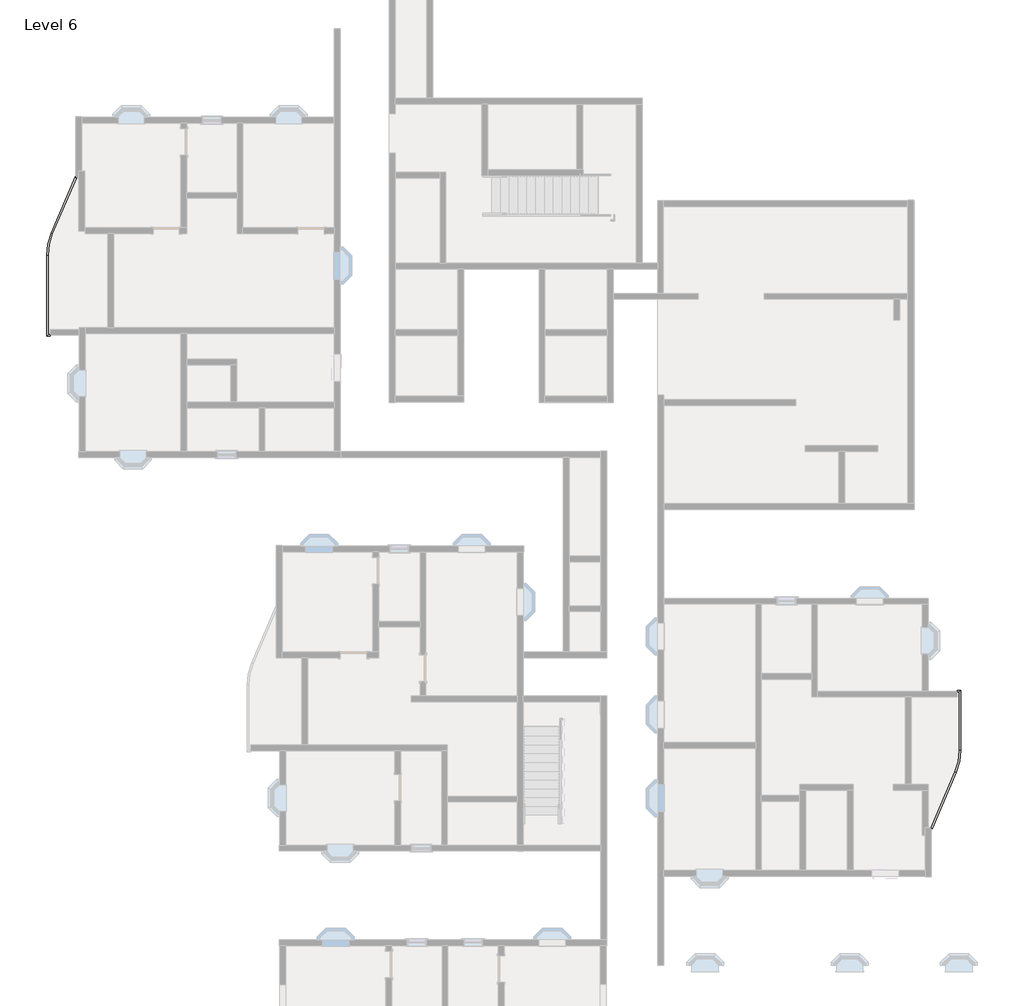
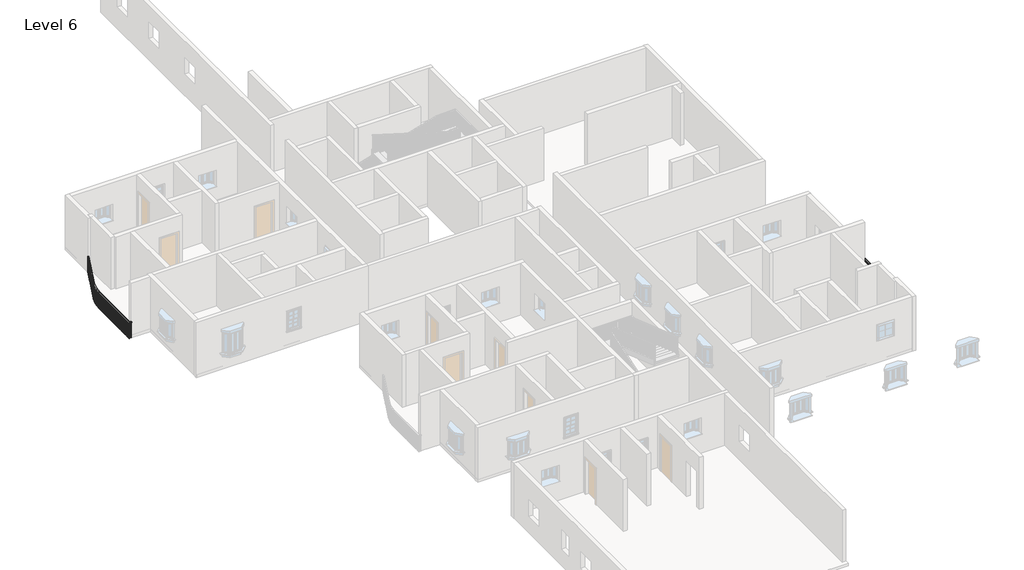
# One storey, part 9 of 14: 2 railings.
"""IFC4 building model written with IfcOpenShell, lengths in millimetres."""

from ifc_helpers import new_model, si_unit, frame, origin, place, context, project, spatial, polyline, circle_curve, outline, extrude, element, save
from ifc_brep_helpers import plane_surface, cylinder_surface, revolved_surface, advanced_brep

model = new_model("IFC4")

# Units and contexts
model_context = context("Model", 3, world=origin())
ifc_project = project(units=[si_unit("LENGTHUNIT", "METRE", prefix="MILLI")], contexts=[model_context])

# Site, building, storey
site = spatial("IfcSite", under=ifc_project)
building = spatial("IfcBuilding", under=site)
storey = spatial("IfcBuildingStorey", under=building, Name="Level 6", Elevation=15240.0)

# Railings
placement = place(None, origin())
element("IfcRailing", 1, ObjectType="Handrail - Rectangular", at=placement, inside=storey, context=model_context, shape_type="SolidModel", body=[
    advanced_brep(
    [(-19327.739878, 12446.0257339, 16154.4), (-19327.739878, 12446.0257339, 16103.6), (-19374.4383922, 12466.022953, 16103.6), (-19374.4383922, 12466.022953, 16154.4), (-20162.483418, 10496.6905323, 16154.4), (-20162.483418, 10496.6905323, 16103.6), (-20209.1819322, 10516.6877514, 16103.6), (-20209.1819322, 10516.6877514, 16154.4), (-20316.2891351, 9746.7948172, 16103.6), (-20316.2891351, 9746.7948172, 16154.4), (-20367.0891351, 9746.7948172, 16103.6), (-20367.0891351, 9746.7948172, 16154.4), (-20316.2891351, 7005.2583494, 16154.4), (-20316.2891351, 7005.2583494, 16103.6), (-20367.0891351, 6954.4583494, 16103.6), (-20367.0891351, 6954.4583494, 16154.4), (-20240.0891351, 7005.2583494, 16154.4), (-20240.0891351, 6954.4583494, 16154.4), (-20240.0891351, 6954.4583494, 16103.6), (-20240.0891351, 7005.2583494, 16103.6)],
    [
        (0, 1),
        (1, 2),
        (2, 3),
        (3, 0),
        (0, 4),
        (4, 5),
        (5, 1),
        (5, 6),
        (6, 2),
        (6, 7),
        (7, 3),
        (7, 4),
        (8, 5, circle_curve(frame((-18411.2891351, 9746.7948172, 16103.6), z_axis=(0.0, 0.0, -1.0), x_axis=(-0.919262090762392, 0.3936460446735823, 0.0)), 1905.0)),
        (4, 9, circle_curve(frame((-18411.2891351, 9746.7948172, 16154.4), z_axis=(0.0, 0.0, 1.0), x_axis=(-0.919262090762392, 0.3936460446735823, 0.0)), 1905.0)),
        (9, 8),
        (10, 6, circle_curve(frame((-18411.2891351, 9746.7948172, 16103.6), z_axis=(0.0, 0.0, -1.0), x_axis=(-0.919262090762392, 0.3936460446735823, 0.0)), 1955.8)),
        (8, 10),
        (11, 7, circle_curve(frame((-18411.2891351, 9746.7948172, 16154.4), z_axis=(0.0, 0.0, -1.0), x_axis=(-0.919262090762392, 0.3936460446735823, 0.0)), 1955.8)),
        (10, 11),
        (11, 9),
        (9, 12),
        (12, 13),
        (13, 8),
        (13, 14),
        (14, 10),
        (14, 15),
        (15, 11),
        (15, 12),
        (16, 17),
        (17, 18),
        (18, 19),
        (19, 16),
        (12, 16),
        (19, 13),
        (18, 14),
        (17, 15),
    ],
    [
        plane_surface(frame((-19351.0891351, 12456.0243434, 16154.4), z_axis=(0.3936460446735829, 0.9192620907623917, 0.0), x_axis=(0.9192620907623917, -0.3936460446735829, 0.0))),
        plane_surface(frame((-19327.739878, 12446.0257339, 16154.4), z_axis=(0.9192620907623915, -0.3936460446735834, 0.0), x_axis=(-0.3936460446735834, -0.9192620907623915, 0.0))),
        plane_surface(frame((-19327.739878, 12446.0257339, 16103.6), z_axis=(0.0, 0.0, -1.0000000000000002), x_axis=(-0.3936460446735834, -0.9192620907623915, 0.0))),
        plane_surface(frame((-19374.4383922, 12466.022953, 16103.6), z_axis=(-0.9192620907623916, 0.393646044673583, 0.0), x_axis=(-0.393646044673583, -0.9192620907623916, 0.0))),
        plane_surface(frame((-19374.4383922, 12466.022953, 16154.4), z_axis=(0.0, 0.0, 1.0), x_axis=(-0.393646044673583, -0.9192620907623916, 0.0))),
        revolved_surface(polyline([(-20162.483418002357, 10496.690532303173, 16154.4), (-20162.483418002357, 10496.690532303173, 16103.6)]), (-18411.2891351, 9746.7948172, 16154.4), (0.0, 0.0, 1.0)),
        plane_surface(frame((-18411.2891351, 9746.7948172, 16103.6), z_axis=(0.0, 0.0, -1.0), x_axis=(-0.919262090762392, 0.3936460446735823, 0.0))),
        cylinder_surface(frame((-18411.2891351, 9746.7948172, 16154.4), z_axis=(0.0, 0.0, 1.0), x_axis=(-0.919262090762392, 0.3936460446735823, 0.0)), 1955.8),
        plane_surface(frame((-18411.2891351, 9746.7948172, 16154.4), z_axis=(0.0, 0.0, 1.0), x_axis=(-0.919262090762392, 0.3936460446735823, 0.0))),
        plane_surface(frame((-20316.2891351, 9746.7948172, 16154.4), z_axis=(1.0, 0.0, 0.0), x_axis=(0.0, -1.0, 0.0))),
        plane_surface(frame((-20316.2891351, 9746.7948172, 16103.6), z_axis=(0.0, 0.0, -1.0), x_axis=(0.0, -1.0, 0.0))),
        plane_surface(frame((-20367.0891351, 9746.7948172, 16103.6), z_axis=(-1.0, 0.0, 0.0), x_axis=(0.0, -1.0, 0.0))),
        plane_surface(frame((-20367.0891351, 9746.7948172, 16154.4), z_axis=(0.0, 0.0, 1.0), x_axis=(0.0, -1.0, 0.0))),
        plane_surface(frame((-20240.0891351, 6979.8583494, 16154.4), z_axis=(1.0, 0.0, 0.0), x_axis=(0.0, 1.0, 0.0))),
        plane_surface(frame((-20316.2891351, 7005.2583494, 16154.4), z_axis=(0.0, 1.0, 0.0), x_axis=(1.0, 0.0, 0.0))),
        plane_surface(frame((-20316.2891351, 7005.2583494, 16103.6), z_axis=(0.0, 0.0, -1.0), x_axis=(1.0, 0.0, 0.0))),
        plane_surface(frame((-20367.0891351, 6954.4583494, 16103.6), z_axis=(0.0, -1.0, 0.0), x_axis=(1.0, 0.0, 0.0))),
        plane_surface(frame((-20367.0891351, 6954.4583494, 16154.4), z_axis=(0.0, 0.0, 1.0), x_axis=(1.0, 0.0, 0.0))),
    ],
    [
        (0, [[1, 2, 3, 4]]),
        (1, [[-1, 5, 6, 7]]),
        (2, [[-2, -7, 8, 9]]),
        (3, [[-3, -9, 10, 11]]),
        (4, [[-4, -11, 12, -5]]),
        (5, [[13, -6, 14, 15]]),
        (6, [[16, -8, -13, 17]]),
        (7, [[18, -10, -16, 19]]),
        (8, [[-14, -12, -18, 20]]),
        (9, [[-15, 21, 22, 23]]),
        (10, [[-17, -23, 24, 25]]),
        (11, [[-19, -25, 26, 27]]),
        (12, [[-20, -27, 28, -21]]),
        (13, [[29, 30, 31, 32]]),
        (14, [[-22, 33, -32, 34]]),
        (15, [[-24, -34, -31, 35]]),
        (16, [[-26, -35, -30, 36]]),
        (17, [[-28, -36, -29, -33]]),
    ],
),
    extrude(outline(polyline([(-20351.2141351, 7013.1198172), (-20332.1641351, 7013.1198172), (-20332.1641351, 6994.0698172), (-20351.2141351, 6994.0698172), (-20351.2141351, 7013.1198172)])), frame((0.0, 0.0, 15240.0), z_axis=(0.0, 0.0, 1.0), x_axis=(1.0, 0.0, 0.0)), (0.0, 0.0, 1.0), 863.6),
    extrude(outline(polyline([(-20351.2141351, 7114.7198172), (-20332.1641351, 7114.7198172), (-20332.1641351, 7095.6698172), (-20351.2141351, 7095.6698172), (-20351.2141351, 7114.7198172)])), frame((0.0, 0.0, 15240.0), z_axis=(0.0, 0.0, 1.0), x_axis=(1.0, 0.0, 0.0)), (0.0, 0.0, 1.0), 863.6),
    extrude(outline(polyline([(-20351.2141351, 7216.3198172), (-20332.1641351, 7216.3198172), (-20332.1641351, 7197.2698172), (-20351.2141351, 7197.2698172), (-20351.2141351, 7216.3198172)])), frame((0.0, 0.0, 15240.0), z_axis=(0.0, 0.0, 1.0), x_axis=(1.0, 0.0, 0.0)), (0.0, 0.0, 1.0), 863.6),
    extrude(outline(polyline([(-20351.2141351, 7317.9198172), (-20332.1641351, 7317.9198172), (-20332.1641351, 7298.8698172), (-20351.2141351, 7298.8698172), (-20351.2141351, 7317.9198172)])), frame((0.0, 0.0, 15240.0), z_axis=(0.0, 0.0, 1.0), x_axis=(1.0, 0.0, 0.0)), (0.0, 0.0, 1.0), 863.6),
    extrude(outline(polyline([(-20351.2141351, 7419.5198172), (-20332.1641351, 7419.5198172), (-20332.1641351, 7400.4698172), (-20351.2141351, 7400.4698172), (-20351.2141351, 7419.5198172)])), frame((0.0, 0.0, 15240.0), z_axis=(0.0, 0.0, 1.0), x_axis=(1.0, 0.0, 0.0)), (0.0, 0.0, 1.0), 863.6),
    extrude(outline(polyline([(-20351.2141351, 7521.1198172), (-20332.1641351, 7521.1198172), (-20332.1641351, 7502.0698172), (-20351.2141351, 7502.0698172), (-20351.2141351, 7521.1198172)])), frame((0.0, 0.0, 15240.0), z_axis=(0.0, 0.0, 1.0), x_axis=(1.0, 0.0, 0.0)), (0.0, 0.0, 1.0), 863.6),
    extrude(outline(polyline([(-20351.2141351, 7622.7198172), (-20332.1641351, 7622.7198172), (-20332.1641351, 7603.6698172), (-20351.2141351, 7603.6698172), (-20351.2141351, 7622.7198172)])), frame((0.0, 0.0, 15240.0), z_axis=(0.0, 0.0, 1.0), x_axis=(1.0, 0.0, 0.0)), (0.0, 0.0, 1.0), 863.6),
    extrude(outline(polyline([(-20351.2141351, 7724.3198172), (-20332.1641351, 7724.3198172), (-20332.1641351, 7705.2698172), (-20351.2141351, 7705.2698172), (-20351.2141351, 7724.3198172)])), frame((0.0, 0.0, 15240.0), z_axis=(0.0, 0.0, 1.0), x_axis=(1.0, 0.0, 0.0)), (0.0, 0.0, 1.0), 863.6),
    extrude(outline(polyline([(-20351.2141351, 7825.9198172), (-20332.1641351, 7825.9198172), (-20332.1641351, 7806.8698172), (-20351.2141351, 7806.8698172), (-20351.2141351, 7825.9198172)])), frame((0.0, 0.0, 15240.0), z_axis=(0.0, 0.0, 1.0), x_axis=(1.0, 0.0, 0.0)), (0.0, 0.0, 1.0), 863.6),
    extrude(outline(polyline([(-20351.2141351, 7927.5198172), (-20332.1641351, 7927.5198172), (-20332.1641351, 7908.4698172), (-20351.2141351, 7908.4698172), (-20351.2141351, 7927.5198172)])), frame((0.0, 0.0, 15240.0), z_axis=(0.0, 0.0, 1.0), x_axis=(1.0, 0.0, 0.0)), (0.0, 0.0, 1.0), 863.6),
    extrude(outline(polyline([(-20351.2141351, 8029.1198172), (-20332.1641351, 8029.1198172), (-20332.1641351, 8010.0698172), (-20351.2141351, 8010.0698172), (-20351.2141351, 8029.1198172)])), frame((0.0, 0.0, 15240.0), z_axis=(0.0, 0.0, 1.0), x_axis=(1.0, 0.0, 0.0)), (0.0, 0.0, 1.0), 863.6),
    extrude(outline(polyline([(-20351.2141351, 8130.7198172), (-20332.1641351, 8130.7198172), (-20332.1641351, 8111.6698172), (-20351.2141351, 8111.6698172), (-20351.2141351, 8130.7198172)])), frame((0.0, 0.0, 15240.0), z_axis=(0.0, 0.0, 1.0), x_axis=(1.0, 0.0, 0.0)), (0.0, 0.0, 1.0), 863.6),
    extrude(outline(polyline([(-20351.2141351, 8232.3198172), (-20332.1641351, 8232.3198172), (-20332.1641351, 8213.2698172), (-20351.2141351, 8213.2698172), (-20351.2141351, 8232.3198172)])), frame((0.0, 0.0, 15240.0), z_axis=(0.0, 0.0, 1.0), x_axis=(1.0, 0.0, 0.0)), (0.0, 0.0, 1.0), 863.6),
    extrude(outline(polyline([(-20351.2141351, 8333.9198172), (-20332.1641351, 8333.9198172), (-20332.1641351, 8314.8698172), (-20351.2141351, 8314.8698172), (-20351.2141351, 8333.9198172)])), frame((0.0, 0.0, 15240.0), z_axis=(0.0, 0.0, 1.0), x_axis=(1.0, 0.0, 0.0)), (0.0, 0.0, 1.0), 863.6),
    extrude(outline(polyline([(-20351.2141351, 8435.5198172), (-20332.1641351, 8435.5198172), (-20332.1641351, 8416.4698172), (-20351.2141351, 8416.4698172), (-20351.2141351, 8435.5198172)])), frame((0.0, 0.0, 15240.0), z_axis=(0.0, 0.0, 1.0), x_axis=(1.0, 0.0, 0.0)), (0.0, 0.0, 1.0), 863.6),
    extrude(outline(polyline([(-20351.2141351, 8537.1198172), (-20332.1641351, 8537.1198172), (-20332.1641351, 8518.0698172), (-20351.2141351, 8518.0698172), (-20351.2141351, 8537.1198172)])), frame((0.0, 0.0, 15240.0), z_axis=(0.0, 0.0, 1.0), x_axis=(1.0, 0.0, 0.0)), (0.0, 0.0, 1.0), 863.6),
    extrude(outline(polyline([(-20351.2141351, 8638.7198172), (-20332.1641351, 8638.7198172), (-20332.1641351, 8619.6698172), (-20351.2141351, 8619.6698172), (-20351.2141351, 8638.7198172)])), frame((0.0, 0.0, 15240.0), z_axis=(0.0, 0.0, 1.0), x_axis=(1.0, 0.0, 0.0)), (0.0, 0.0, 1.0), 863.6),
    extrude(outline(polyline([(-20351.2141351, 8740.3198172), (-20332.1641351, 8740.3198172), (-20332.1641351, 8721.2698172), (-20351.2141351, 8721.2698172), (-20351.2141351, 8740.3198172)])), frame((0.0, 0.0, 15240.0), z_axis=(0.0, 0.0, 1.0), x_axis=(1.0, 0.0, 0.0)), (0.0, 0.0, 1.0), 863.6),
    extrude(outline(polyline([(-20351.2141351, 8841.9198172), (-20332.1641351, 8841.9198172), (-20332.1641351, 8822.8698172), (-20351.2141351, 8822.8698172), (-20351.2141351, 8841.9198172)])), frame((0.0, 0.0, 15240.0), z_axis=(0.0, 0.0, 1.0), x_axis=(1.0, 0.0, 0.0)), (0.0, 0.0, 1.0), 863.6),
    extrude(outline(polyline([(-20351.2141351, 8943.5198172), (-20332.1641351, 8943.5198172), (-20332.1641351, 8924.4698172), (-20351.2141351, 8924.4698172), (-20351.2141351, 8943.5198172)])), frame((0.0, 0.0, 15240.0), z_axis=(0.0, 0.0, 1.0), x_axis=(1.0, 0.0, 0.0)), (0.0, 0.0, 1.0), 863.6),
    extrude(outline(polyline([(-20351.2141351, 9045.1198172), (-20332.1641351, 9045.1198172), (-20332.1641351, 9026.0698172), (-20351.2141351, 9026.0698172), (-20351.2141351, 9045.1198172)])), frame((0.0, 0.0, 15240.0), z_axis=(0.0, 0.0, 1.0), x_axis=(1.0, 0.0, 0.0)), (0.0, 0.0, 1.0), 863.6),
    extrude(outline(polyline([(-20351.2141351, 9146.7198172), (-20332.1641351, 9146.7198172), (-20332.1641351, 9127.6698172), (-20351.2141351, 9127.6698172), (-20351.2141351, 9146.7198172)])), frame((0.0, 0.0, 15240.0), z_axis=(0.0, 0.0, 1.0), x_axis=(1.0, 0.0, 0.0)), (0.0, 0.0, 1.0), 863.6),
    extrude(outline(polyline([(-20351.2141351, 9248.3198172), (-20332.1641351, 9248.3198172), (-20332.1641351, 9229.2698172), (-20351.2141351, 9229.2698172), (-20351.2141351, 9248.3198172)])), frame((0.0, 0.0, 15240.0), z_axis=(0.0, 0.0, 1.0), x_axis=(1.0, 0.0, 0.0)), (0.0, 0.0, 1.0), 863.6),
    extrude(outline(polyline([(-20351.2141351, 9349.9198172), (-20332.1641351, 9349.9198172), (-20332.1641351, 9330.8698172), (-20351.2141351, 9330.8698172), (-20351.2141351, 9349.9198172)])), frame((0.0, 0.0, 15240.0), z_axis=(0.0, 0.0, 1.0), x_axis=(1.0, 0.0, 0.0)), (0.0, 0.0, 1.0), 863.6),
    extrude(outline(polyline([(-20351.2141351, 9451.5198172), (-20332.1641351, 9451.5198172), (-20332.1641351, 9432.4698172), (-20351.2141351, 9432.4698172), (-20351.2141351, 9451.5198172)])), frame((0.0, 0.0, 15240.0), z_axis=(0.0, 0.0, 1.0), x_axis=(1.0, 0.0, 0.0)), (0.0, 0.0, 1.0), 863.6),
    extrude(outline(polyline([(-20351.2141351, 9553.1198172), (-20332.1641351, 9553.1198172), (-20332.1641351, 9534.0698172), (-20351.2141351, 9534.0698172), (-20351.2141351, 9553.1198172)])), frame((0.0, 0.0, 15240.0), z_axis=(0.0, 0.0, 1.0), x_axis=(1.0, 0.0, 0.0)), (0.0, 0.0, 1.0), 863.6),
    extrude(outline(polyline([(-20351.2141351, 9654.7198172), (-20332.1641351, 9654.7198172), (-20332.1641351, 9635.6698172), (-20351.2141351, 9635.6698172), (-20351.2141351, 9654.7198172)])), frame((0.0, 0.0, 15240.0), z_axis=(0.0, 0.0, 1.0), x_axis=(1.0, 0.0, 0.0)), (0.0, 0.0, 1.0), 863.6),
    extrude(outline(polyline([(-20349.6005818, 9826.4720848), (-20330.5630441, 9825.7831307), (-20331.2519982, 9806.745593), (-20350.289536, 9807.4345471), (-20349.6005818, 9826.4720848)])), frame((0.0, 0.0, 15240.0), z_axis=(0.0, 0.0, 1.0), x_axis=(1.0, 0.0, 0.0)), (0.0, 0.0, 1.0), 863.6),
    extrude(outline(polyline([(-20342.724955, 9928.3310534), (-20323.750023, 9926.6415402), (-20325.4395363, 9907.6666081), (-20344.4144683, 9909.3561214), (-20342.724955, 9928.3310534)])), frame((0.0, 0.0, 15240.0), z_axis=(0.0, 0.0, 1.0), x_axis=(1.0, 0.0, 0.0)), (0.0, 0.0, 1.0), 863.6),
    extrude(outline(polyline([(-20330.5003254, 10029.6872677), (-20311.6405491, 10027.0018743), (-20314.3259425, 10008.142098), (-20333.1857188, 10010.8274914), (-20330.5003254, 10029.6872677)])), frame((0.0, 0.0, 15240.0), z_axis=(0.0, 0.0, 1.0), x_axis=(1.0, 0.0, 0.0)), (0.0, 0.0, 1.0), 863.6),
    extrude(outline(polyline([(-20312.9605484, 10130.2600272), (-20294.2681589, 10126.5861907), (-20297.9419954, 10107.8938012), (-20316.6343849, 10111.5676377), (-20312.9605484, 10130.2600272)])), frame((0.0, 0.0, 15240.0), z_axis=(0.0, 0.0, 1.0), x_axis=(1.0, 0.0, 0.0)), (0.0, 0.0, 1.0), 863.6),
    extrude(outline(polyline([(-20290.1541995, 10229.7708014), (-20271.6809643, 10225.1186963), (-20276.3330693, 10206.6454611), (-20294.8063045, 10211.2975662), (-20290.1541995, 10229.7708014)])), frame((0.0, 0.0, 15240.0), z_axis=(0.0, 0.0, 1.0), x_axis=(1.0, 0.0, 0.0)), (0.0, 0.0, 1.0), 863.6),
    extrude(outline(polyline([(-20262.1444395, 10327.9440008), (-20243.9415192, 10322.3265109), (-20249.5590091, 10304.1235906), (-20267.7619294, 10309.7410805), (-20262.1444395, 10327.9440008)])), frame((0.0, 0.0, 15240.0), z_axis=(0.0, 0.0, 1.0), x_axis=(1.0, 0.0, 0.0)), (0.0, 0.0, 1.0), 863.6),
    extrude(outline(polyline([(-20229.0088399, 10424.5077402), (-20211.1266465, 10417.9404228), (-20217.693964, 10400.0582293), (-20235.5761574, 10406.6255468), (-20229.0088399, 10424.5077402)])), frame((0.0, 0.0, 15240.0), z_axis=(0.0, 0.0, 1.0), x_axis=(1.0, 0.0, 0.0)), (0.0, 0.0, 1.0), 863.6),
    extrude(outline(polyline([(-20155.9843907, 10600.589225), (-20138.4724479, 10593.0902678), (-20145.9714051, 10575.578325), (-20163.4833479, 10583.0772822), (-20155.9843907, 10600.589225)])), frame((0.0, 0.0, 15240.0), z_axis=(0.0, 0.0, 1.0), x_axis=(1.0, 0.0, 0.0)), (0.0, 0.0, 1.0), 863.6),
    extrude(outline(polyline([(-20115.9899526, 10693.9862534), (-20098.4780098, 10686.4872963), (-20105.9769669, 10668.9753534), (-20123.4889098, 10676.4743106), (-20115.9899526, 10693.9862534)])), frame((0.0, 0.0, 15240.0), z_axis=(0.0, 0.0, 1.0), x_axis=(1.0, 0.0, 0.0)), (0.0, 0.0, 1.0), 863.6),
    extrude(outline(polyline([(-20075.9955145, 10787.3832818), (-20058.4835716, 10779.8843247), (-20065.9825288, 10762.3723818), (-20083.4944716, 10769.871339), (-20075.9955145, 10787.3832818)])), frame((0.0, 0.0, 15240.0), z_axis=(0.0, 0.0, 1.0), x_axis=(1.0, 0.0, 0.0)), (0.0, 0.0, 1.0), 863.6),
    extrude(outline(polyline([(-20036.0010763, 10880.7803103), (-20018.4891335, 10873.2813531), (-20025.9880906, 10855.7694103), (-20043.5000335, 10863.2683674), (-20036.0010763, 10880.7803103)])), frame((0.0, 0.0, 15240.0), z_axis=(0.0, 0.0, 1.0), x_axis=(1.0, 0.0, 0.0)), (0.0, 0.0, 1.0), 863.6),
    extrude(outline(polyline([(-19996.0066382, 10974.1773387), (-19978.4946954, 10966.6783815), (-19985.9936525, 10949.1664387), (-20003.5055953, 10956.6653958), (-19996.0066382, 10974.1773387)])), frame((0.0, 0.0, 15240.0), z_axis=(0.0, 0.0, 1.0), x_axis=(1.0, 0.0, 0.0)), (0.0, 0.0, 1.0), 863.6),
    extrude(outline(polyline([(-19956.0122, 11067.5743671), (-19938.5002572, 11060.0754099), (-19945.9992144, 11042.5634671), (-19963.5111572, 11050.0624243), (-19956.0122, 11067.5743671)])), frame((0.0, 0.0, 15240.0), z_axis=(0.0, 0.0, 1.0), x_axis=(1.0, 0.0, 0.0)), (0.0, 0.0, 1.0), 863.6),
    extrude(outline(polyline([(-19916.0177619, 11160.9713955), (-19898.5058191, 11153.4724384), (-19906.0047762, 11135.9604955), (-19923.5167191, 11143.4594527), (-19916.0177619, 11160.9713955)])), frame((0.0, 0.0, 15240.0), z_axis=(0.0, 0.0, 1.0), x_axis=(1.0, 0.0, 0.0)), (0.0, 0.0, 1.0), 863.6),
    extrude(outline(polyline([(-19876.0233238, 11254.3684239), (-19858.5113809, 11246.8694668), (-19866.0103381, 11229.357524), (-19883.5222809, 11236.8564811), (-19876.0233238, 11254.3684239)])), frame((0.0, 0.0, 15240.0), z_axis=(0.0, 0.0, 1.0), x_axis=(1.0, 0.0, 0.0)), (0.0, 0.0, 1.0), 863.6),
    extrude(outline(polyline([(-19836.0288856, 11347.7654524), (-19818.5169428, 11340.2664952), (-19826.0159, 11322.7545524), (-19843.5278428, 11330.2535095), (-19836.0288856, 11347.7654524)])), frame((0.0, 0.0, 15240.0), z_axis=(0.0, 0.0, 1.0), x_axis=(1.0, 0.0, 0.0)), (0.0, 0.0, 1.0), 863.6),
    extrude(outline(polyline([(-19796.0344475, 11441.1624808), (-19778.5225047, 11433.6635236), (-19786.0214618, 11416.1515808), (-19803.5334046, 11423.650538), (-19796.0344475, 11441.1624808)])), frame((0.0, 0.0, 15240.0), z_axis=(0.0, 0.0, 1.0), x_axis=(1.0, 0.0, 0.0)), (0.0, 0.0, 1.0), 863.6),
    extrude(outline(polyline([(-19756.0400094, 11534.5595092), (-19738.5280665, 11527.060552), (-19746.0270237, 11509.5486092), (-19763.5389665, 11517.0475664), (-19756.0400094, 11534.5595092)])), frame((0.0, 0.0, 15240.0), z_axis=(0.0, 0.0, 1.0), x_axis=(1.0, 0.0, 0.0)), (0.0, 0.0, 1.0), 863.6),
    extrude(outline(polyline([(-19716.0455712, 11627.9565376), (-19698.5336284, 11620.4575805), (-19706.0325855, 11602.9456376), (-19723.5445284, 11610.4445948), (-19716.0455712, 11627.9565376)])), frame((0.0, 0.0, 15240.0), z_axis=(0.0, 0.0, 1.0), x_axis=(1.0, 0.0, 0.0)), (0.0, 0.0, 1.0), 863.6),
    extrude(outline(polyline([(-19676.0511331, 11721.353566), (-19658.5391902, 11713.8546089), (-19666.0381474, 11696.3426661), (-19683.5500902, 11703.8416232), (-19676.0511331, 11721.353566)])), frame((0.0, 0.0, 15240.0), z_axis=(0.0, 0.0, 1.0), x_axis=(1.0, 0.0, 0.0)), (0.0, 0.0, 1.0), 863.6),
    extrude(outline(polyline([(-19636.0566949, 11814.7505945), (-19618.5447521, 11807.2516373), (-19626.0437093, 11789.7396945), (-19643.5556521, 11797.2386516), (-19636.0566949, 11814.7505945)])), frame((0.0, 0.0, 15240.0), z_axis=(0.0, 0.0, 1.0), x_axis=(1.0, 0.0, 0.0)), (0.0, 0.0, 1.0), 863.6),
    extrude(outline(polyline([(-19596.0622568, 11908.1476229), (-19578.550314, 11900.6486657), (-19586.0492711, 11883.1367229), (-19603.561214, 11890.6356801), (-19596.0622568, 11908.1476229)])), frame((0.0, 0.0, 15240.0), z_axis=(0.0, 0.0, 1.0), x_axis=(1.0, 0.0, 0.0)), (0.0, 0.0, 1.0), 863.6),
    extrude(outline(polyline([(-19556.0678187, 12001.5446513), (-19538.5558758, 11994.0456942), (-19546.054833, 11976.5337513), (-19563.5667758, 11984.0327085), (-19556.0678187, 12001.5446513)])), frame((0.0, 0.0, 15240.0), z_axis=(0.0, 0.0, 1.0), x_axis=(1.0, 0.0, 0.0)), (0.0, 0.0, 1.0), 863.6),
    extrude(outline(polyline([(-19516.0733805, 12094.9416797), (-19498.5614377, 12087.4427226), (-19506.0603948, 12069.9307797), (-19523.5723377, 12077.4297369), (-19516.0733805, 12094.9416797)])), frame((0.0, 0.0, 15240.0), z_axis=(0.0, 0.0, 1.0), x_axis=(1.0, 0.0, 0.0)), (0.0, 0.0, 1.0), 863.6),
    extrude(outline(polyline([(-19476.0789424, 12188.3387082), (-19458.5669996, 12180.839751), (-19466.0659567, 12163.3278082), (-19483.5778995, 12170.8267653), (-19476.0789424, 12188.3387082)])), frame((0.0, 0.0, 15240.0), z_axis=(0.0, 0.0, 1.0), x_axis=(1.0, 0.0, 0.0)), (0.0, 0.0, 1.0), 863.6),
    extrude(outline(polyline([(-19436.0845042, 12281.7357366), (-19418.5725614, 12274.2367794), (-19426.0715186, 12256.7248366), (-19443.5834614, 12264.2237937), (-19436.0845042, 12281.7357366)])), frame((0.0, 0.0, 15240.0), z_axis=(0.0, 0.0, 1.0), x_axis=(1.0, 0.0, 0.0)), (0.0, 0.0, 1.0), 863.6),
    extrude(outline(polyline([(-19396.0900661, 12375.132765), (-19378.5781233, 12367.6338078), (-19386.0770804, 12350.121865), (-19403.5890233, 12357.6208222), (-19396.0900661, 12375.132765)])), frame((0.0, 0.0, 15240.0), z_axis=(0.0, 0.0, 1.0), x_axis=(1.0, 0.0, 0.0)), (0.0, 0.0, 1.0), 863.6),
    extrude(outline(polyline([(-20351.2141351, 6989.3833494), (-20332.1641351, 6989.3833494), (-20332.1641351, 6970.3333494), (-20351.2141351, 6970.3333494), (-20351.2141351, 6989.3833494)])), frame((0.0, 0.0, 15240.0), z_axis=(0.0, 0.0, 1.0), x_axis=(1.0, 0.0, 0.0)), (0.0, 0.0, 1.0), 863.6),
    extrude(outline(polyline([(-20351.2141351, 9756.3198172), (-20332.1641351, 9756.3198172), (-20332.1641351, 9737.2698172), (-20351.2141351, 9737.2698172), (-20351.2141351, 9756.3198172)])), frame((0.0, 0.0, 15240.0), z_axis=(0.0, 0.0, 1.0), x_axis=(1.0, 0.0, 0.0)), (0.0, 0.0, 1.0), 863.6),
    extrude(outline(polyline([(-20190.839168, 10519.1945919), (-20173.3272251, 10511.6956347), (-20180.8261823, 10494.1836919), (-20198.3381251, 10501.682649), (-20190.839168, 10519.1945919)])), frame((0.0, 0.0, 15240.0), z_axis=(0.0, 0.0, 1.0), x_axis=(1.0, 0.0, 0.0)), (0.0, 0.0, 1.0), 863.6),
    extrude(outline(polyline([(-20259.1391351, 6970.3333494), (-20259.1391351, 6989.3833494), (-20240.0891351, 6989.3833494), (-20240.0891351, 6970.3333494), (-20259.1391351, 6970.3333494)])), frame((0.0, 0.0, 15240.0), z_axis=(0.0, 0.0, 1.0), x_axis=(1.0, 0.0, 0.0)), (0.0, 0.0, 1.0), 863.6),
    extrude(outline(polyline([(-19359.8451065, 12459.773822), (-19342.3331637, 12452.2748648), (-19349.8321209, 12434.762922), (-19367.3440637, 12442.2618792), (-19359.8451065, 12459.773822)])), frame((0.0, 0.0, 15240.0), z_axis=(0.0, 0.0, 1.0), x_axis=(1.0, 0.0, 0.0)), (0.0, 0.0, 1.0), 863.6),
])
element("IfcRailing", 2, ObjectType="Handrail - Rectangular", at=placement, inside=storey, context=model_context, shape_type="SolidModel", body=[
    advanced_brep(
    [(10250.7887952, -10096.81198, 16154.4), (10250.7887952, -10096.81198, 16103.6), (10297.4873094, -10116.8091991, 16103.6), (10297.4873094, -10116.8091991, 16154.4), (11085.5323352, -8147.4767784, 16154.4), (11085.5323352, -8147.4767784, 16103.6), (11132.2308494, -8167.4739975, 16103.6), (11132.2308494, -8167.4739975, 16154.4), (11239.3380523, -7397.5810633, 16103.6), (11239.3380523, -7397.5810633, 16154.4), (11290.1380523, -7397.5810633, 16103.6), (11290.1380523, -7397.5810633, 16154.4), (11239.3380523, -5378.0542694, 16154.4), (11239.3380523, -5378.0542694, 16103.6), (11290.1380523, -5327.2542694, 16103.6), (11290.1380523, -5327.2542694, 16154.4), (11163.1380523, -5378.0542694, 16154.4), (11163.1380523, -5327.2542694, 16154.4), (11163.1380523, -5327.2542694, 16103.6), (11163.1380523, -5378.0542694, 16103.6)],
    [
        (0, 1),
        (1, 2),
        (2, 3),
        (3, 0),
        (0, 4),
        (4, 5),
        (5, 1),
        (5, 6),
        (6, 2),
        (6, 7),
        (7, 3),
        (7, 4),
        (8, 5, circle_curve(frame((9334.3380523, -7397.5810633, 16103.6), z_axis=(0.0, 0.0, -1.0), x_axis=(0.9192620907624003, -0.3936460446735628, 0.0)), 1905.0)),
        (4, 9, circle_curve(frame((9334.3380523, -7397.5810633, 16154.4), z_axis=(0.0, 0.0, 1.0), x_axis=(0.9192620907624003, -0.3936460446735628, 0.0)), 1905.0)),
        (9, 8),
        (10, 6, circle_curve(frame((9334.3380523, -7397.5810633, 16103.6), z_axis=(0.0, 0.0, -1.0), x_axis=(0.9192620907624003, -0.3936460446735628, 0.0)), 1955.8)),
        (8, 10),
        (11, 7, circle_curve(frame((9334.3380523, -7397.5810633, 16154.4), z_axis=(0.0, 0.0, -1.0), x_axis=(0.9192620907624003, -0.3936460446735628, 0.0)), 1955.8)),
        (10, 11),
        (11, 9),
        (9, 12),
        (12, 13),
        (13, 8),
        (13, 14),
        (14, 10),
        (14, 15),
        (15, 11),
        (15, 12),
        (16, 17),
        (17, 18),
        (18, 19),
        (19, 16),
        (12, 16),
        (19, 13),
        (18, 14),
        (17, 15),
    ],
    [
        plane_surface(frame((10274.1380523, -10106.8105895, 16154.4), z_axis=(-0.3936460446735629, -0.9192620907624003, 0.0), x_axis=(0.9192620907624003, -0.3936460446735629, 0.0))),
        plane_surface(frame((10250.7887952, -10096.81198, 16154.4), z_axis=(-0.9192620907624005, 0.39364604467356235, 0.0), x_axis=(0.39364604467356235, 0.9192620907624005, 0.0))),
        plane_surface(frame((10250.7887952, -10096.81198, 16103.6), z_axis=(0.0, 0.0, -1.0), x_axis=(0.39364604467356235, 0.9192620907624005, 0.0))),
        plane_surface(frame((10297.4873094, -10116.8091991, 16103.6), z_axis=(0.9192620907624003, -0.3936460446735627, 0.0), x_axis=(0.3936460446735627, 0.9192620907624003, 0.0))),
        plane_surface(frame((10297.4873094, -10116.8091991, 16154.4), z_axis=(0.0, 0.0, 1.0), x_axis=(0.3936460446735627, 0.9192620907624003, 0.0))),
        revolved_surface(polyline([(11085.532335202372, -8147.476778403137, 16154.4), (11085.532335202372, -8147.476778403137, 16103.6)]), (9334.3380523, -7397.5810633, 16154.4), (0.0, 0.0, 1.0)),
        plane_surface(frame((9334.3380523, -7397.5810633, 16103.6), z_axis=(0.0, 0.0, -1.0), x_axis=(0.9192620907624003, -0.3936460446735628, 0.0))),
        cylinder_surface(frame((9334.3380523, -7397.5810633, 16154.4), z_axis=(0.0, 0.0, 1.0), x_axis=(0.9192620907624003, -0.3936460446735628, 0.0)), 1955.8),
        plane_surface(frame((9334.3380523, -7397.5810633, 16154.4), z_axis=(0.0, 0.0, 1.0), x_axis=(0.9192620907624003, -0.3936460446735628, 0.0))),
        plane_surface(frame((11239.3380523, -7397.5810633, 16154.4), z_axis=(-1.0, 0.0, 0.0), x_axis=(0.0, 1.0, 0.0))),
        plane_surface(frame((11239.3380523, -7397.5810633, 16103.6), z_axis=(0.0, 0.0, -1.0), x_axis=(0.0, 1.0, 0.0))),
        plane_surface(frame((11290.1380523, -7397.5810633, 16103.6), z_axis=(1.0, 0.0, 0.0), x_axis=(0.0, 1.0, 0.0))),
        plane_surface(frame((11290.1380523, -7397.5810633, 16154.4), z_axis=(0.0, 0.0, 1.0), x_axis=(0.0, 1.0, 0.0))),
        plane_surface(frame((11163.1380523, -5352.6542694, 16154.4), z_axis=(-1.0, 0.0, 0.0), x_axis=(0.0, -1.0, 0.0))),
        plane_surface(frame((11239.3380523, -5378.0542694, 16154.4), z_axis=(0.0, -1.0, 0.0), x_axis=(-1.0, 0.0, 0.0))),
        plane_surface(frame((11239.3380523, -5378.0542694, 16103.6), z_axis=(0.0, 0.0, -1.0), x_axis=(-1.0, 0.0, 0.0))),
        plane_surface(frame((11290.1380523, -5327.2542694, 16103.6), z_axis=(0.0, 1.0, 0.0), x_axis=(-1.0, 0.0, 0.0))),
        plane_surface(frame((11290.1380523, -5327.2542694, 16154.4), z_axis=(0.0, 0.0, 1.0), x_axis=(-1.0, 0.0, 0.0))),
    ],
    [
        (0, [[1, 2, 3, 4]]),
        (1, [[-1, 5, 6, 7]]),
        (2, [[-2, -7, 8, 9]]),
        (3, [[-3, -9, 10, 11]]),
        (4, [[-4, -11, 12, -5]]),
        (5, [[13, -6, 14, 15]]),
        (6, [[16, -8, -13, 17]]),
        (7, [[18, -10, -16, 19]]),
        (8, [[-14, -12, -18, 20]]),
        (9, [[-15, 21, 22, 23]]),
        (10, [[-17, -23, 24, 25]]),
        (11, [[-19, -25, 26, 27]]),
        (12, [[-20, -27, 28, -21]]),
        (13, [[29, 30, 31, 32]]),
        (14, [[-22, 33, -32, 34]]),
        (15, [[-24, -34, -31, 35]]),
        (16, [[-26, -35, -30, 36]]),
        (17, [[-28, -36, -29, -33]]),
    ],
),
    extrude(outline(polyline([(11274.2630523, -5375.1060633), (11255.2130523, -5375.1060633), (11255.2130523, -5356.0560633), (11274.2630523, -5356.0560633), (11274.2630523, -5375.1060633)])), frame((0.0, 0.0, 15240.0), z_axis=(0.0, 0.0, 1.0), x_axis=(1.0, 0.0, 0.0)), (0.0, 0.0, 1.0), 863.6),
    extrude(outline(polyline([(11274.2630523, -5476.7060633), (11255.2130523, -5476.7060633), (11255.2130523, -5457.6560633), (11274.2630523, -5457.6560633), (11274.2630523, -5476.7060633)])), frame((0.0, 0.0, 15240.0), z_axis=(0.0, 0.0, 1.0), x_axis=(1.0, 0.0, 0.0)), (0.0, 0.0, 1.0), 863.6),
    extrude(outline(polyline([(11274.2630523, -5578.3060633), (11255.2130523, -5578.3060633), (11255.2130523, -5559.2560633), (11274.2630523, -5559.2560633), (11274.2630523, -5578.3060633)])), frame((0.0, 0.0, 15240.0), z_axis=(0.0, 0.0, 1.0), x_axis=(1.0, 0.0, 0.0)), (0.0, 0.0, 1.0), 863.6),
    extrude(outline(polyline([(11274.2630523, -5679.9060633), (11255.2130523, -5679.9060633), (11255.2130523, -5660.8560633), (11274.2630523, -5660.8560633), (11274.2630523, -5679.9060633)])), frame((0.0, 0.0, 15240.0), z_axis=(0.0, 0.0, 1.0), x_axis=(1.0, 0.0, 0.0)), (0.0, 0.0, 1.0), 863.6),
    extrude(outline(polyline([(11274.2630523, -5781.5060633), (11255.2130523, -5781.5060633), (11255.2130523, -5762.4560633), (11274.2630523, -5762.4560633), (11274.2630523, -5781.5060633)])), frame((0.0, 0.0, 15240.0), z_axis=(0.0, 0.0, 1.0), x_axis=(1.0, 0.0, 0.0)), (0.0, 0.0, 1.0), 863.6),
    extrude(outline(polyline([(11274.2630523, -5883.1060633), (11255.2130523, -5883.1060633), (11255.2130523, -5864.0560633), (11274.2630523, -5864.0560633), (11274.2630523, -5883.1060633)])), frame((0.0, 0.0, 15240.0), z_axis=(0.0, 0.0, 1.0), x_axis=(1.0, 0.0, 0.0)), (0.0, 0.0, 1.0), 863.6),
    extrude(outline(polyline([(11274.2630523, -5984.7060633), (11255.2130523, -5984.7060633), (11255.2130523, -5965.6560633), (11274.2630523, -5965.6560633), (11274.2630523, -5984.7060633)])), frame((0.0, 0.0, 15240.0), z_axis=(0.0, 0.0, 1.0), x_axis=(1.0, 0.0, 0.0)), (0.0, 0.0, 1.0), 863.6),
    extrude(outline(polyline([(11274.2630523, -6086.3060633), (11255.2130523, -6086.3060633), (11255.2130523, -6067.2560633), (11274.2630523, -6067.2560633), (11274.2630523, -6086.3060633)])), frame((0.0, 0.0, 15240.0), z_axis=(0.0, 0.0, 1.0), x_axis=(1.0, 0.0, 0.0)), (0.0, 0.0, 1.0), 863.6),
    extrude(outline(polyline([(11274.2630523, -6187.9060633), (11255.2130523, -6187.9060633), (11255.2130523, -6168.8560633), (11274.2630523, -6168.8560633), (11274.2630523, -6187.9060633)])), frame((0.0, 0.0, 15240.0), z_axis=(0.0, 0.0, 1.0), x_axis=(1.0, 0.0, 0.0)), (0.0, 0.0, 1.0), 863.6),
    extrude(outline(polyline([(11274.2630523, -6289.5060633), (11255.2130523, -6289.5060633), (11255.2130523, -6270.4560633), (11274.2630523, -6270.4560633), (11274.2630523, -6289.5060633)])), frame((0.0, 0.0, 15240.0), z_axis=(0.0, 0.0, 1.0), x_axis=(1.0, 0.0, 0.0)), (0.0, 0.0, 1.0), 863.6),
    extrude(outline(polyline([(11274.2630523, -6391.1060633), (11255.2130523, -6391.1060633), (11255.2130523, -6372.0560633), (11274.2630523, -6372.0560633), (11274.2630523, -6391.1060633)])), frame((0.0, 0.0, 15240.0), z_axis=(0.0, 0.0, 1.0), x_axis=(1.0, 0.0, 0.0)), (0.0, 0.0, 1.0), 863.6),
    extrude(outline(polyline([(11274.2630523, -6492.7060633), (11255.2130523, -6492.7060633), (11255.2130523, -6473.6560633), (11274.2630523, -6473.6560633), (11274.2630523, -6492.7060633)])), frame((0.0, 0.0, 15240.0), z_axis=(0.0, 0.0, 1.0), x_axis=(1.0, 0.0, 0.0)), (0.0, 0.0, 1.0), 863.6),
    extrude(outline(polyline([(11274.2630523, -6594.3060633), (11255.2130523, -6594.3060633), (11255.2130523, -6575.2560633), (11274.2630523, -6575.2560633), (11274.2630523, -6594.3060633)])), frame((0.0, 0.0, 15240.0), z_axis=(0.0, 0.0, 1.0), x_axis=(1.0, 0.0, 0.0)), (0.0, 0.0, 1.0), 863.6),
    extrude(outline(polyline([(11274.2630523, -6695.9060633), (11255.2130523, -6695.9060633), (11255.2130523, -6676.8560633), (11274.2630523, -6676.8560633), (11274.2630523, -6695.9060633)])), frame((0.0, 0.0, 15240.0), z_axis=(0.0, 0.0, 1.0), x_axis=(1.0, 0.0, 0.0)), (0.0, 0.0, 1.0), 863.6),
    extrude(outline(polyline([(11274.2630523, -6797.5060633), (11255.2130523, -6797.5060633), (11255.2130523, -6778.4560633), (11274.2630523, -6778.4560633), (11274.2630523, -6797.5060633)])), frame((0.0, 0.0, 15240.0), z_axis=(0.0, 0.0, 1.0), x_axis=(1.0, 0.0, 0.0)), (0.0, 0.0, 1.0), 863.6),
    extrude(outline(polyline([(11274.2630523, -6899.1060633), (11255.2130523, -6899.1060633), (11255.2130523, -6880.0560633), (11274.2630523, -6880.0560633), (11274.2630523, -6899.1060633)])), frame((0.0, 0.0, 15240.0), z_axis=(0.0, 0.0, 1.0), x_axis=(1.0, 0.0, 0.0)), (0.0, 0.0, 1.0), 863.6),
    extrude(outline(polyline([(11274.2630523, -7000.7060633), (11255.2130523, -7000.7060633), (11255.2130523, -6981.6560633), (11274.2630523, -6981.6560633), (11274.2630523, -7000.7060633)])), frame((0.0, 0.0, 15240.0), z_axis=(0.0, 0.0, 1.0), x_axis=(1.0, 0.0, 0.0)), (0.0, 0.0, 1.0), 863.6),
    extrude(outline(polyline([(11274.2630523, -7102.3060633), (11255.2130523, -7102.3060633), (11255.2130523, -7083.2560633), (11274.2630523, -7083.2560633), (11274.2630523, -7102.3060633)])), frame((0.0, 0.0, 15240.0), z_axis=(0.0, 0.0, 1.0), x_axis=(1.0, 0.0, 0.0)), (0.0, 0.0, 1.0), 863.6),
    extrude(outline(polyline([(11274.2630523, -7203.9060633), (11255.2130523, -7203.9060633), (11255.2130523, -7184.8560633), (11274.2630523, -7184.8560633), (11274.2630523, -7203.9060633)])), frame((0.0, 0.0, 15240.0), z_axis=(0.0, 0.0, 1.0), x_axis=(1.0, 0.0, 0.0)), (0.0, 0.0, 1.0), 863.6),
    extrude(outline(polyline([(11274.2630523, -7305.5060633), (11255.2130523, -7305.5060633), (11255.2130523, -7286.4560633), (11274.2630523, -7286.4560633), (11274.2630523, -7305.5060633)])), frame((0.0, 0.0, 15240.0), z_axis=(0.0, 0.0, 1.0), x_axis=(1.0, 0.0, 0.0)), (0.0, 0.0, 1.0), 863.6),
    extrude(outline(polyline([(11272.649499, -7477.2583309), (11253.6119612, -7476.5693768), (11254.3009154, -7457.531839), (11273.3384531, -7458.2207932), (11272.649499, -7477.2583309)])), frame((0.0, 0.0, 15240.0), z_axis=(0.0, 0.0, 1.0), x_axis=(1.0, 0.0, 0.0)), (0.0, 0.0, 1.0), 863.6),
    extrude(outline(polyline([(11265.7738721, -7579.1172995), (11246.7989401, -7577.4277862), (11248.4884534, -7558.4528542), (11267.4633854, -7560.1423675), (11265.7738721, -7579.1172995)])), frame((0.0, 0.0, 15240.0), z_axis=(0.0, 0.0, 1.0), x_axis=(1.0, 0.0, 0.0)), (0.0, 0.0, 1.0), 863.6),
    extrude(outline(polyline([(11253.5492425, -7680.4735138), (11234.6894662, -7677.7881204), (11237.3748596, -7658.9283441), (11256.2346359, -7661.6137375), (11253.5492425, -7680.4735138)])), frame((0.0, 0.0, 15240.0), z_axis=(0.0, 0.0, 1.0), x_axis=(1.0, 0.0, 0.0)), (0.0, 0.0, 1.0), 863.6),
    extrude(outline(polyline([(11236.0094655, -7781.0462733), (11217.317076, -7777.3724368), (11220.9909125, -7758.6800473), (11239.683302, -7762.3538838), (11236.0094655, -7781.0462733)])), frame((0.0, 0.0, 15240.0), z_axis=(0.0, 0.0, 1.0), x_axis=(1.0, 0.0, 0.0)), (0.0, 0.0, 1.0), 863.6),
    extrude(outline(polyline([(11213.2031166, -7880.5570475), (11194.7298814, -7875.9049424), (11199.3819865, -7857.4317072), (11217.8552217, -7862.0838123), (11213.2031166, -7880.5570475)])), frame((0.0, 0.0, 15240.0), z_axis=(0.0, 0.0, 1.0), x_axis=(1.0, 0.0, 0.0)), (0.0, 0.0, 1.0), 863.6),
    extrude(outline(polyline([(11185.1933567, -7978.7302469), (11166.9904364, -7973.1127569), (11172.6079263, -7954.9098367), (11190.8108466, -7960.5273266), (11185.1933567, -7978.7302469)])), frame((0.0, 0.0, 15240.0), z_axis=(0.0, 0.0, 1.0), x_axis=(1.0, 0.0, 0.0)), (0.0, 0.0, 1.0), 863.6),
    extrude(outline(polyline([(11152.0577571, -8075.2939863), (11134.1755637, -8068.7266689), (11140.7428811, -8050.8444754), (11158.6250745, -8057.4117929), (11152.0577571, -8075.2939863)])), frame((0.0, 0.0, 15240.0), z_axis=(0.0, 0.0, 1.0), x_axis=(1.0, 0.0, 0.0)), (0.0, 0.0, 1.0), 863.6),
    extrude(outline(polyline([(11079.0333079, -8251.3754711), (11061.5213651, -8243.8765139), (11069.0203222, -8226.3645711), (11086.5322651, -8233.8635283), (11079.0333079, -8251.3754711)])), frame((0.0, 0.0, 15240.0), z_axis=(0.0, 0.0, 1.0), x_axis=(1.0, 0.0, 0.0)), (0.0, 0.0, 1.0), 863.6),
    extrude(outline(polyline([(11039.0388698, -8344.7724995), (11021.5269269, -8337.2735424), (11029.0258841, -8319.7615995), (11046.5378269, -8327.2605567), (11039.0388698, -8344.7724995)])), frame((0.0, 0.0, 15240.0), z_axis=(0.0, 0.0, 1.0), x_axis=(1.0, 0.0, 0.0)), (0.0, 0.0, 1.0), 863.6),
    extrude(outline(polyline([(10999.0444316, -8438.1695279), (10981.5324888, -8430.6705708), (10989.0314459, -8413.1586279), (11006.5433888, -8420.6575851), (10999.0444316, -8438.1695279)])), frame((0.0, 0.0, 15240.0), z_axis=(0.0, 0.0, 1.0), x_axis=(1.0, 0.0, 0.0)), (0.0, 0.0, 1.0), 863.6),
    extrude(outline(polyline([(10959.0499935, -8531.5665563), (10941.5380507, -8524.0675992), (10949.0370078, -8506.5556564), (10966.5489506, -8514.0546135), (10959.0499935, -8531.5665563)])), frame((0.0, 0.0, 15240.0), z_axis=(0.0, 0.0, 1.0), x_axis=(1.0, 0.0, 0.0)), (0.0, 0.0, 1.0), 863.6),
    extrude(outline(polyline([(10919.0555553, -8624.9635848), (10901.5436125, -8617.4646276), (10909.0425697, -8599.9526848), (10926.5545125, -8607.4516419), (10919.0555553, -8624.9635848)])), frame((0.0, 0.0, 15240.0), z_axis=(0.0, 0.0, 1.0), x_axis=(1.0, 0.0, 0.0)), (0.0, 0.0, 1.0), 863.6),
    extrude(outline(polyline([(10879.0611172, -8718.3606132), (10861.5491744, -8710.861656), (10869.0481315, -8693.3497132), (10886.5600744, -8700.8486704), (10879.0611172, -8718.3606132)])), frame((0.0, 0.0, 15240.0), z_axis=(0.0, 0.0, 1.0), x_axis=(1.0, 0.0, 0.0)), (0.0, 0.0, 1.0), 863.6),
    extrude(outline(polyline([(10839.0666791, -8811.7576416), (10821.5547362, -8804.2586845), (10829.0536934, -8786.7467416), (10846.5656362, -8794.2456988), (10839.0666791, -8811.7576416)])), frame((0.0, 0.0, 15240.0), z_axis=(0.0, 0.0, 1.0), x_axis=(1.0, 0.0, 0.0)), (0.0, 0.0, 1.0), 863.6),
    extrude(outline(polyline([(10799.0722409, -8905.15467), (10781.5602981, -8897.6557129), (10789.0592553, -8880.1437701), (10806.5711981, -8887.6427272), (10799.0722409, -8905.15467)])), frame((0.0, 0.0, 15240.0), z_axis=(0.0, 0.0, 1.0), x_axis=(1.0, 0.0, 0.0)), (0.0, 0.0, 1.0), 863.6),
    extrude(outline(polyline([(10759.0778028, -8998.5516985), (10741.56586, -8991.0527413), (10749.0648171, -8973.5407985), (10766.5767599, -8981.0397556), (10759.0778028, -8998.5516985)])), frame((0.0, 0.0, 15240.0), z_axis=(0.0, 0.0, 1.0), x_axis=(1.0, 0.0, 0.0)), (0.0, 0.0, 1.0), 863.6),
    extrude(outline(polyline([(10719.0833647, -9091.9487269), (10701.5714218, -9084.4497697), (10709.070379, -9066.9378269), (10726.5823218, -9074.436784), (10719.0833647, -9091.9487269)])), frame((0.0, 0.0, 15240.0), z_axis=(0.0, 0.0, 1.0), x_axis=(1.0, 0.0, 0.0)), (0.0, 0.0, 1.0), 863.6),
    extrude(outline(polyline([(10679.0889265, -9185.3457553), (10661.5769837, -9177.8467981), (10669.0759408, -9160.3348553), (10686.5878837, -9167.8338125), (10679.0889265, -9185.3457553)])), frame((0.0, 0.0, 15240.0), z_axis=(0.0, 0.0, 1.0), x_axis=(1.0, 0.0, 0.0)), (0.0, 0.0, 1.0), 863.6),
    extrude(outline(polyline([(10639.0944884, -9278.7427837), (10621.5825455, -9271.2438266), (10629.0815027, -9253.7318837), (10646.5934455, -9261.2308409), (10639.0944884, -9278.7427837)])), frame((0.0, 0.0, 15240.0), z_axis=(0.0, 0.0, 1.0), x_axis=(1.0, 0.0, 0.0)), (0.0, 0.0, 1.0), 863.6),
    extrude(outline(polyline([(10599.1000502, -9372.1398121), (10581.5881074, -9364.640855), (10589.0870646, -9347.1289122), (10606.5990074, -9354.6278693), (10599.1000502, -9372.1398121)])), frame((0.0, 0.0, 15240.0), z_axis=(0.0, 0.0, 1.0), x_axis=(1.0, 0.0, 0.0)), (0.0, 0.0, 1.0), 863.6),
    extrude(outline(polyline([(10559.1056121, -9465.5368406), (10541.5936693, -9458.0378834), (10549.0926264, -9440.5259406), (10566.6045693, -9448.0248977), (10559.1056121, -9465.5368406)])), frame((0.0, 0.0, 15240.0), z_axis=(0.0, 0.0, 1.0), x_axis=(1.0, 0.0, 0.0)), (0.0, 0.0, 1.0), 863.6),
    extrude(outline(polyline([(10519.111174, -9558.933869), (10501.5992311, -9551.4349118), (10509.0981883, -9533.922969), (10526.6101311, -9541.4219262), (10519.111174, -9558.933869)])), frame((0.0, 0.0, 15240.0), z_axis=(0.0, 0.0, 1.0), x_axis=(1.0, 0.0, 0.0)), (0.0, 0.0, 1.0), 863.6),
    extrude(outline(polyline([(10479.1167358, -9652.3308974), (10461.604793, -9644.8319403), (10469.1037501, -9627.3199974), (10486.615693, -9634.8189546), (10479.1167358, -9652.3308974)])), frame((0.0, 0.0, 15240.0), z_axis=(0.0, 0.0, 1.0), x_axis=(1.0, 0.0, 0.0)), (0.0, 0.0, 1.0), 863.6),
    extrude(outline(polyline([(10439.1222977, -9745.7279258), (10421.6103549, -9738.2289687), (10429.109312, -9720.7170258), (10446.6212548, -9728.215983), (10439.1222977, -9745.7279258)])), frame((0.0, 0.0, 15240.0), z_axis=(0.0, 0.0, 1.0), x_axis=(1.0, 0.0, 0.0)), (0.0, 0.0, 1.0), 863.6),
    extrude(outline(polyline([(10399.1278595, -9839.1249542), (10381.6159167, -9831.6259971), (10389.1148739, -9814.1140543), (10406.6268167, -9821.6130114), (10399.1278595, -9839.1249542)])), frame((0.0, 0.0, 15240.0), z_axis=(0.0, 0.0, 1.0), x_axis=(1.0, 0.0, 0.0)), (0.0, 0.0, 1.0), 863.6),
    extrude(outline(polyline([(10359.1334214, -9932.5219827), (10341.6214786, -9925.0230255), (10349.1204357, -9907.5110827), (10366.6323786, -9915.0100398), (10359.1334214, -9932.5219827)])), frame((0.0, 0.0, 15240.0), z_axis=(0.0, 0.0, 1.0), x_axis=(1.0, 0.0, 0.0)), (0.0, 0.0, 1.0), 863.6),
    extrude(outline(polyline([(10319.1389833, -10025.9190111), (10301.6270404, -10018.4200539), (10309.1259976, -10000.9081111), (10326.6379404, -10008.4070683), (10319.1389833, -10025.9190111)])), frame((0.0, 0.0, 15240.0), z_axis=(0.0, 0.0, 1.0), x_axis=(1.0, 0.0, 0.0)), (0.0, 0.0, 1.0), 863.6),
    extrude(outline(polyline([(11274.2630523, -5362.1792694), (11255.2130523, -5362.1792694), (11255.2130523, -5343.1292694), (11274.2630523, -5343.1292694), (11274.2630523, -5362.1792694)])), frame((0.0, 0.0, 15240.0), z_axis=(0.0, 0.0, 1.0), x_axis=(1.0, 0.0, 0.0)), (0.0, 0.0, 1.0), 863.6),
    extrude(outline(polyline([(11274.2630523, -7407.1060633), (11255.2130523, -7407.1060633), (11255.2130523, -7388.0560633), (11274.2630523, -7388.0560633), (11274.2630523, -7407.1060633)])), frame((0.0, 0.0, 15240.0), z_axis=(0.0, 0.0, 1.0), x_axis=(1.0, 0.0, 0.0)), (0.0, 0.0, 1.0), 863.6),
    extrude(outline(polyline([(11113.8880851, -8169.9808379), (11096.3761423, -8162.4818808), (11103.8750995, -8144.969938), (11121.3870423, -8152.4688951), (11113.8880851, -8169.9808379)])), frame((0.0, 0.0, 15240.0), z_axis=(0.0, 0.0, 1.0), x_axis=(1.0, 0.0, 0.0)), (0.0, 0.0, 1.0), 863.6),
    extrude(outline(polyline([(11182.1880523, -5343.1292694), (11182.1880523, -5362.1792694), (11163.1380523, -5362.1792694), (11163.1380523, -5343.1292694), (11182.1880523, -5343.1292694)])), frame((0.0, 0.0, 15240.0), z_axis=(0.0, 0.0, 1.0), x_axis=(1.0, 0.0, 0.0)), (0.0, 0.0, 1.0), 863.6),
    extrude(outline(polyline([(10282.8940237, -10110.5600681), (10265.3820809, -10103.0611109), (10272.881038, -10085.5491681), (10290.3929809, -10093.0481253), (10282.8940237, -10110.5600681)])), frame((0.0, 0.0, 15240.0), z_axis=(0.0, 0.0, 1.0), x_axis=(1.0, 0.0, 0.0)), (0.0, 0.0, 1.0), 863.6),
])

save(model, "model.ifc")

# Revit data of these elements
# Type "Handrail - Rectangular"
#   Assembly Code = "C2010400"
#   built-in parameter 1008612 = 0.0416667 (stored number, unit not read)
#   built-in parameter 1008611 = 0.0416667 (stored number, unit not read)
#   built-in parameter 1008609 = 0.333333 (stored number, unit not read)
#   built-in parameter 1008604 = 0.166667 (stored number, unit not read)
#   built-in parameter 1008603 = 0.166667 (stored number, unit not read)
#   Railing Height = 3' - 0"
#   built-in parameter 1008630 = 2
#   built-in parameter 1008610 = 2
#   built-in parameter 1008618 = Baluster - Square : 3/4"
# Elements 1, 2 (IfcRailing, "Handrail - Rectangular")
#   Phase Created = New Construction
